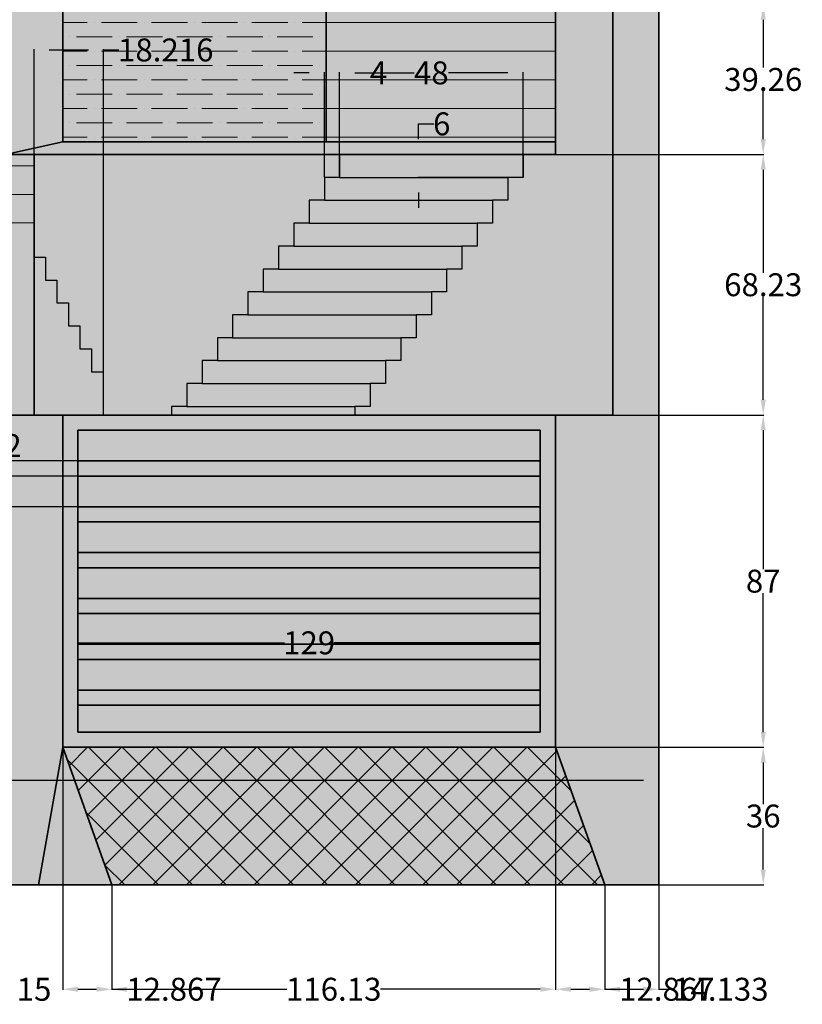
# Model space of a CAD drawing. Units: inches. Extents: x 184 to 649, y 215 to 818.
# Tile 3 of 9: x 442 to 647, y 215 to 473. Entities that reach past the tile are written whole.
import ezdxf

# ---------------------------------------------------------------- set-up
doc = ezdxf.new("R2010")
doc.units = ezdxf.units.IN
doc.header["$MEASUREMENT"] = 0
for name, color, linetype, lineweight in [('A-ANNO-DIMS', 2, 'Continuous', 18), ('A-ELEV', 7, 'Continuous', 35), ('A-ELEV-FILL', 9, 'Continuous', 13), ('A-ELEV-PATT', 8, 'Continuous', 13), ('A-FLOR-STRS', 3, 'Continuous', 25)]:
    doc.layers.add(name, color=color, linetype=linetype, lineweight=lineweight)
doc.styles.get("Standard").update_dxf_attribs({"font": 'arial.ttf'})
doc.dimstyles.get("Standard").update_dxf_attribs({"dimtxt": 6, "dimasz": 4, "dimexe": 0.18, "dimexo": 0.0625, "dimgap": 0.09, "dimtad": 0, "dimtih": 1, "dimtoh": 1, "dimdec": 0, "dimzin": 0, "dimdsep": 46, "dimlunit": 3, "dimtxsty": 'Standard', "dimcen": 0.09, "dimadec": 0, "dimazin": 0, "dimtfac": 1, "dimtdec": 0, "dimtofl": 0, "dimtmove": 0, "dimatfit": 3, "dimfxl": 1, "dimtolj": 1, "dimtzin": 0, "dimarcsym": 0})

# ---------------------------------------------------------------- blocks, each defined once
blk = doc.blocks.new('*D9')
at = {"layer": 'A-ANNO-DIMS', "color": 0, "lineweight": -2, "transparency": 16777216}
for p, q in [((248.97, 246.79), (248.97, 274.26)), ((252.97, 274.08), (422.27, 274.08)), ((604.97, 274.08), (435.68, 274.08)), ((608.97, 246.79), (608.97, 274.26))]:
    blk.add_line(p, q, dxfattribs=at)
at = {"layer": 'A-ANNO-DIMS', "color": 0, "transparency": 16777216}
for points in [[(252.97, 274.74), (252.97, 273.41), (248.97, 274.08)], [(604.97, 274.74), (604.97, 273.41), (608.97, 274.08)]]:
    blk.add_solid(points, dxfattribs=at)
at = {"layer": 'Defpoints', "color": 0, "transparency": 16777216}
for p in [(608.97, 274.08), (248.97, 246.73), (608.97, 246.73)]:
    blk.add_point(p, dxfattribs=at)
at = {"layer": 'A-ANNO-DIMS', "color": 0, "transparency": 16777216, "insert": (428.97, 274.08), "char_height": 6, "attachment_point": 5}
blk.add_mtext('\\A1;360', dxfattribs=at)
blk = doc.blocks.new('*D14')
at = {"layer": 'A-ANNO-DIMS', "color": 0, "lineweight": -2, "transparency": 16777216}
for p, q in [((452.97, 282.66), (452.97, 219.2)), ((437.97, 246.66), (437.97, 219.2)), ((433.97, 219.38), (429.97, 219.38)), ((456.97, 219.38), (460.97, 219.38))]:
    blk.add_line(p, q, dxfattribs=at)
at = {"layer": 'A-ANNO-DIMS', "color": 0, "transparency": 16777216}
for points in [[(433.97, 220.04), (433.97, 218.71), (437.97, 219.38)], [(456.97, 220.04), (456.97, 218.71), (452.97, 219.38)]]:
    blk.add_solid(points, dxfattribs=at)
at = {"layer": 'Defpoints', "color": 0, "transparency": 16777216}
for p in [(452.97, 282.73), (437.97, 246.73), (452.97, 219.38)]:
    blk.add_point(p, dxfattribs=at)
at = {"layer": 'A-ANNO-DIMS', "color": 0, "transparency": 16777216, "insert": (445.47, 219.38), "char_height": 6, "attachment_point": 5}
blk.add_mtext('\\A1;15', dxfattribs=at)
blk = doc.blocks.new('*D15')
at = {"layer": 'A-ANNO-DIMS', "color": 0, "lineweight": -2, "transparency": 16777216}
for p, q in [((452.97, 282.66), (452.97, 219.2)), ((465.84, 246.66), (465.84, 219.2)), ((456.97, 219.38), (461.84, 219.38)), ((465.84, 219.38), (469.84, 219.38))]:
    blk.add_line(p, q, dxfattribs=at)
at = {"layer": 'A-ANNO-DIMS', "color": 0, "transparency": 16777216}
for points in [[(456.97, 220.04), (456.97, 218.71), (452.97, 219.38)], [(461.84, 220.04), (461.84, 218.71), (465.84, 219.38)]]:
    blk.add_solid(points, dxfattribs=at)
at = {"layer": 'Defpoints', "color": 0, "transparency": 16777216}
for p in [(452.97, 282.73), (465.84, 246.73), (465.84, 219.38)]:
    blk.add_point(p, dxfattribs=at)
at = {"layer": 'A-ANNO-DIMS', "color": 0, "transparency": 16777216, "insert": (482.1, 219.38), "char_height": 6, "attachment_point": 5}
blk.add_mtext('\\A1;12.867', dxfattribs=at)
blk = doc.blocks.new('*D16')
at = {"layer": 'A-ANNO-DIMS', "color": 0, "lineweight": -2, "transparency": 16777216}
for p, q in [((581.97, 282.66), (581.97, 219.2)), ((465.84, 246.66), (465.84, 219.2)), ((469.84, 219.38), (511.64, 219.38)), ((577.97, 219.38), (536.17, 219.38))]:
    blk.add_line(p, q, dxfattribs=at)
at = {"layer": 'A-ANNO-DIMS', "color": 0, "transparency": 16777216}
for points in [[(469.84, 220.04), (469.84, 218.71), (465.84, 219.38)], [(577.97, 220.04), (577.97, 218.71), (581.97, 219.38)]]:
    blk.add_solid(points, dxfattribs=at)
at = {"layer": 'Defpoints', "color": 0, "transparency": 16777216}
for p in [(581.97, 282.73), (465.84, 246.73), (581.97, 219.38)]:
    blk.add_point(p, dxfattribs=at)
at = {"layer": 'A-ANNO-DIMS', "color": 0, "transparency": 16777216, "insert": (523.91, 219.38), "char_height": 6, "attachment_point": 5}
blk.add_mtext('\\A1;116.13', dxfattribs=at)
blk = doc.blocks.new('*D17')
at = {"layer": 'A-ANNO-DIMS', "color": 0, "lineweight": -2, "transparency": 16777216}
for p, q in [((581.97, 282.66), (581.97, 219.2)), ((594.84, 246.66), (594.84, 219.2)), ((585.97, 219.38), (590.84, 219.38)), ((594.84, 219.38), (598.84, 219.38))]:
    blk.add_line(p, q, dxfattribs=at)
at = {"layer": 'A-ANNO-DIMS', "color": 0, "transparency": 16777216}
for points in [[(585.97, 220.04), (585.97, 218.71), (581.97, 219.38)], [(590.84, 220.04), (590.84, 218.71), (594.84, 219.38)]]:
    blk.add_solid(points, dxfattribs=at)
at = {"layer": 'Defpoints', "color": 0, "transparency": 16777216}
for p in [(581.97, 282.73), (594.84, 246.73), (594.84, 219.38)]:
    blk.add_point(p, dxfattribs=at)
at = {"layer": 'A-ANNO-DIMS', "color": 0, "transparency": 16777216, "insert": (611.1, 219.38), "char_height": 6, "attachment_point": 5}
blk.add_mtext('\\A1;12.867', dxfattribs=at)
blk = doc.blocks.new('*D18')
at = {"layer": 'A-ANNO-DIMS', "color": 0, "lineweight": -2, "transparency": 16777216}
for p, q in [((594.84, 246.66), (594.84, 219.2)), ((608.97, 246.66), (608.97, 219.2)), ((598.84, 219.38), (604.97, 219.38)), ((608.97, 219.38), (612.97, 219.38))]:
    blk.add_line(p, q, dxfattribs=at)
at = {"layer": 'A-ANNO-DIMS', "color": 0, "transparency": 16777216}
for points in [[(598.84, 220.04), (598.84, 218.71), (594.84, 219.38)], [(604.97, 220.04), (604.97, 218.71), (608.97, 219.38)]]:
    blk.add_solid(points, dxfattribs=at)
at = {"layer": 'Defpoints', "color": 0, "transparency": 16777216}
for p in [(594.84, 246.73), (608.97, 246.73), (608.97, 219.38)]:
    blk.add_point(p, dxfattribs=at)
at = {"layer": 'A-ANNO-DIMS', "color": 0, "transparency": 16777216, "insert": (625.23, 219.38), "char_height": 6, "attachment_point": 5}
blk.add_mtext('\\A1;14.133', dxfattribs=at)
blk = doc.blocks.new('*D44')
at = {"layer": 'A-ANNO-DIMS', "color": 0, "lineweight": -2, "transparency": 16777216}
for p, q in [((582.04, 282.73), (636.5, 282.73)), ((636.32, 278.73), (636.32, 267.88)), ((636.32, 250.73), (636.32, 261.57)), ((594.9, 246.73), (636.5, 246.73))]:
    blk.add_line(p, q, dxfattribs=at)
at = {"layer": 'A-ANNO-DIMS', "color": 0, "transparency": 16777216}
for points in [[(635.66, 278.73), (636.99, 278.73), (636.32, 282.73)], [(635.66, 250.73), (636.99, 250.73), (636.32, 246.73)]]:
    blk.add_solid(points, dxfattribs=at)
at = {"layer": 'Defpoints', "color": 0, "transparency": 16777216}
for p in [(581.97, 282.73), (636.32, 282.73), (594.84, 246.73)]:
    blk.add_point(p, dxfattribs=at)
at = {"layer": 'A-ANNO-DIMS', "color": 0, "transparency": 16777216, "insert": (636.32, 264.73), "char_height": 6, "attachment_point": 5}
blk.add_mtext('\\A1;36', dxfattribs=at)
blk = doc.blocks.new('*D45')
at = {"layer": 'A-ANNO-DIMS', "color": 0, "lineweight": -2, "transparency": 16777216}
for p, q in [((582.04, 369.73), (636.5, 369.73)), ((636.32, 365.73), (636.32, 329.38)), ((636.32, 286.73), (636.32, 323.07)), ((582.04, 282.73), (636.5, 282.73))]:
    blk.add_line(p, q, dxfattribs=at)
at = {"layer": 'A-ANNO-DIMS', "color": 0, "transparency": 16777216}
for points in [[(635.66, 365.73), (636.99, 365.73), (636.32, 369.73)], [(635.66, 286.73), (636.99, 286.73), (636.32, 282.73)]]:
    blk.add_solid(points, dxfattribs=at)
at = {"layer": 'Defpoints', "color": 0, "transparency": 16777216}
for p in [(581.97, 369.73), (636.32, 369.73), (581.97, 282.73)]:
    blk.add_point(p, dxfattribs=at)
at = {"layer": 'A-ANNO-DIMS', "color": 0, "transparency": 16777216, "insert": (636.32, 326.23), "char_height": 6, "attachment_point": 5}
blk.add_mtext('\\A1;87', dxfattribs=at)
blk = doc.blocks.new('*D46')
at = {"layer": 'A-ANNO-DIMS', "color": 0, "lineweight": -2, "transparency": 16777216}
for p, q in [((582.04, 437.96), (636.5, 437.96)), ((636.32, 433.96), (636.32, 407)), ((636.32, 373.73), (636.32, 400.69)), ((582.04, 369.73), (636.5, 369.73))]:
    blk.add_line(p, q, dxfattribs=at)
at = {"layer": 'A-ANNO-DIMS', "color": 0, "transparency": 16777216}
for points in [[(635.66, 433.96), (636.99, 433.96), (636.32, 437.96)], [(635.66, 373.73), (636.99, 373.73), (636.32, 369.73)]]:
    blk.add_solid(points, dxfattribs=at)
at = {"layer": 'Defpoints', "color": 0, "transparency": 16777216}
for p in [(581.97, 437.96), (636.32, 437.96), (581.97, 369.73)]:
    blk.add_point(p, dxfattribs=at)
at = {"layer": 'A-ANNO-DIMS', "color": 0, "transparency": 16777216, "insert": (636.32, 403.84), "char_height": 6, "attachment_point": 5}
blk.add_mtext('\\A1;68.23', dxfattribs=at)
blk = doc.blocks.new('*D47')
at = {"layer": 'A-ANNO-DIMS', "color": 0, "lineweight": -2, "transparency": 16777216}
for p, q in [((561.04, 477.22), (636.5, 477.22)), ((636.32, 473.22), (636.32, 460.75)), ((636.32, 441.96), (636.32, 454.44)), ((582.04, 437.96), (636.5, 437.96))]:
    blk.add_line(p, q, dxfattribs=at)
at = {"layer": 'A-ANNO-DIMS', "color": 0, "transparency": 16777216}
for points in [[(635.66, 473.22), (636.99, 473.22), (636.32, 477.22)], [(635.66, 441.96), (636.99, 441.96), (636.32, 437.96)]]:
    blk.add_solid(points, dxfattribs=at)
at = {"layer": 'Defpoints', "color": 0, "transparency": 16777216}
for p in [(560.97, 477.22), (636.32, 477.22), (581.97, 437.96)]:
    blk.add_point(p, dxfattribs=at)
at = {"layer": 'A-ANNO-DIMS', "color": 0, "transparency": 16777216, "insert": (636.32, 457.59), "char_height": 6, "attachment_point": 5}
blk.add_mtext('\\A1;39.26', dxfattribs=at)
blk = doc.blocks.new('*D64')
at = {"layer": 'A-ANNO-DIMS', "color": 0, "lineweight": -2, "transparency": 16777216}
for p, q in [((445.47, 438.02), (445.47, 465.49)), ((449.47, 465.31), (459.69, 465.31)), ((463.69, 438.02), (463.69, 465.49)), ((463.69, 465.31), (467.69, 465.31))]:
    blk.add_line(p, q, dxfattribs=at)
at = {"layer": 'A-ANNO-DIMS', "color": 0, "transparency": 16777216}
for points in [[(449.47, 465.98), (449.47, 464.64), (445.47, 465.31)], [(459.69, 465.98), (459.69, 464.64), (463.69, 465.31)]]:
    blk.add_solid(points, dxfattribs=at)
at = {"layer": 'Defpoints', "color": 0, "transparency": 16777216}
for p in [(463.69, 465.31), (445.47, 437.96), (463.69, 437.96)]:
    blk.add_point(p, dxfattribs=at)
at = {"layer": 'A-ANNO-DIMS', "color": 0, "transparency": 16777216, "insert": (479.95, 465.31), "char_height": 6, "attachment_point": 5}
blk.add_mtext('\\A1;18.216', dxfattribs=at)
blk = doc.blocks.new('*D65')
at = {"layer": 'A-ANNO-DIMS', "color": 0, "lineweight": -2, "transparency": 16777216}
for p, q in [((525.46, 432.02), (525.46, 459.49)), ((529.46, 459.31), (544.94, 459.31)), ((569.46, 459.31), (553.97, 459.31)), ((573.46, 432.02), (573.46, 459.49))]:
    blk.add_line(p, q, dxfattribs=at)
at = {"layer": 'A-ANNO-DIMS', "color": 0, "transparency": 16777216}
for points in [[(529.46, 459.98), (529.46, 458.64), (525.46, 459.31)], [(569.46, 459.98), (569.46, 458.64), (573.46, 459.31)]]:
    blk.add_solid(points, dxfattribs=at)
at = {"layer": 'Defpoints', "color": 0, "transparency": 16777216}
for p in [(573.46, 459.31), (525.46, 431.96), (573.46, 431.96)]:
    blk.add_point(p, dxfattribs=at)
at = {"layer": 'A-ANNO-DIMS', "color": 0, "transparency": 16777216, "insert": (549.46, 459.31), "char_height": 6, "attachment_point": 5}
blk.add_mtext('\\A1;48', dxfattribs=at)
blk = doc.blocks.new('*D66')
at = {"layer": 'A-ANNO-DIMS', "color": 0, "lineweight": -2, "transparency": 16777216}
for p, q in [((517.46, 459.31), (513.46, 459.31)), ((521.46, 432.02), (521.46, 459.49)), ((525.46, 432.02), (525.46, 459.49)), ((529.46, 459.31), (533.46, 459.31))]:
    blk.add_line(p, q, dxfattribs=at)
at = {"layer": 'A-ANNO-DIMS', "color": 0, "transparency": 16777216}
for points in [[(517.46, 459.98), (517.46, 458.64), (521.46, 459.31)], [(529.46, 459.98), (529.46, 458.64), (525.46, 459.31)]]:
    blk.add_solid(points, dxfattribs=at)
at = {"layer": 'Defpoints', "color": 0, "transparency": 16777216}
for p in [(525.46, 459.31), (521.46, 431.96), (525.46, 431.96)]:
    blk.add_point(p, dxfattribs=at)
at = {"layer": 'A-ANNO-DIMS', "color": 0, "transparency": 16777216, "insert": (535.62, 459.31), "char_height": 6, "attachment_point": 5}
blk.add_mtext('\\A1;4', dxfattribs=at)
blk = doc.blocks.new('*D67')
at = {"layer": 'A-ANNO-DIMS', "color": 0, "lineweight": -2, "transparency": 16777216}
for p, q in [((546.11, 441.96), (546.11, 445.96)), ((546.11, 445.96), (550.11, 445.96)), ((573.4, 437.96), (545.93, 437.96)), ((573.4, 431.96), (545.93, 431.96)), ((546.11, 427.96), (546.11, 423.96))]:
    blk.add_line(p, q, dxfattribs=at)
at = {"layer": 'A-ANNO-DIMS', "color": 0, "transparency": 16777216}
for points in [[(545.44, 441.96), (546.77, 441.96), (546.11, 437.96)], [(545.44, 427.96), (546.77, 427.96), (546.11, 431.96)]]:
    blk.add_solid(points, dxfattribs=at)
at = {"layer": 'Defpoints', "color": 0, "transparency": 16777216}
for p in [(546.11, 437.96), (573.46, 437.96), (573.46, 431.96)]:
    blk.add_point(p, dxfattribs=at)
at = {"layer": 'A-ANNO-DIMS', "color": 0, "transparency": 16777216, "insert": (552.18, 445.96), "char_height": 6, "attachment_point": 5}
blk.add_mtext('\\A1;6', dxfattribs=at)
blk = doc.blocks.new('*D70')
at = {"layer": 'A-ANNO-DIMS', "color": 0, "lineweight": -2, "transparency": 16777216}
for p, q in [((452.97, 282.79), (452.97, 310.26)), ((456.97, 310.08), (511.03, 310.08)), ((577.97, 310.08), (523.91, 310.08)), ((581.97, 282.79), (581.97, 310.26))]:
    blk.add_line(p, q, dxfattribs=at)
at = {"layer": 'A-ANNO-DIMS', "color": 0, "transparency": 16777216}
for points in [[(456.97, 310.74), (456.97, 309.41), (452.97, 310.08)], [(577.97, 310.74), (577.97, 309.41), (581.97, 310.08)]]:
    blk.add_solid(points, dxfattribs=at)
at = {"layer": 'Defpoints', "color": 0, "transparency": 16777216}
for p in [(581.97, 310.08), (452.97, 282.73), (581.97, 282.73)]:
    blk.add_point(p, dxfattribs=at)
at = {"layer": 'A-ANNO-DIMS', "color": 0, "transparency": 16777216, "insert": (517.47, 310.08), "char_height": 6, "attachment_point": 5}
blk.add_mtext('\\A1;129', dxfattribs=at)
blk = doc.blocks.new('*D71')
at = {"layer": 'A-ANNO-DIMS', "color": 0, "lineweight": -2, "transparency": 16777216}
for p, q in [((429.62, 361.73), (429.62, 365.73)), ((429.62, 365.73), (433.62, 365.73)), ((456.91, 357.73), (429.44, 357.73)), ((456.91, 353.73), (429.44, 353.73)), ((429.62, 349.73), (429.62, 345.73))]:
    blk.add_line(p, q, dxfattribs=at)
at = {"layer": 'A-ANNO-DIMS', "color": 0, "transparency": 16777216}
for points in [[(428.96, 361.73), (430.29, 361.73), (429.62, 357.73)], [(428.96, 349.73), (430.29, 349.73), (429.62, 353.73)]]:
    blk.add_solid(points, dxfattribs=at)
at = {"layer": 'Defpoints', "color": 0, "transparency": 16777216}
for p in [(429.62, 357.73), (456.97, 357.73), (456.97, 353.73)]:
    blk.add_point(p, dxfattribs=at)
at = {"layer": 'A-ANNO-DIMS', "color": 0, "transparency": 16777216, "insert": (435.79, 365.73), "char_height": 6, "attachment_point": 5}
blk.add_mtext('\\A1;4', dxfattribs=at)
blk = doc.blocks.new('*D72')
at = {"layer": 'A-ANNO-DIMS', "color": 0, "lineweight": -2, "transparency": 16777216}
for p, q in [((429.62, 357.73), (429.62, 361.73)), ((429.62, 361.73), (433.62, 361.73)), ((456.91, 357.73), (429.44, 357.73)), ((429.62, 349.73), (429.62, 353.73)), ((456.91, 345.73), (429.44, 345.73))]:
    blk.add_line(p, q, dxfattribs=at)
at = {"layer": 'A-ANNO-DIMS', "color": 0, "transparency": 16777216}
for points in [[(428.96, 353.73), (430.29, 353.73), (429.62, 357.73)], [(428.96, 349.73), (430.29, 349.73), (429.62, 345.73)]]:
    blk.add_solid(points, dxfattribs=at)
at = {"layer": 'Defpoints', "color": 0, "transparency": 16777216}
for p in [(429.62, 357.73), (456.97, 357.73), (456.97, 345.73)]:
    blk.add_point(p, dxfattribs=at)
at = {"layer": 'A-ANNO-DIMS', "color": 0, "transparency": 16777216, "insert": (437.7, 361.73), "char_height": 6, "attachment_point": 5}
blk.add_mtext('\\A1;12', dxfattribs=at)

msp = doc.modelspace()

# ---------------------------------------------------------------- hatches: boundary and pattern name
at = {"layer": 'A-ELEV-FILL'}
h = msp.add_hatch(color=256, dxfattribs=at)
h.dxf.hatch_style = 1
h.paths.add_polyline_path([(452.9726, 369.7265), (248.9726, 369.7265), (248.9726, 246.7265), (275.9726, 246.7265), (275.9726, 328.7265), (437.9726, 328.7265), (437.9726, 246.7265), (446.6666, 246.7265), (452.9726, 282.7265)])
h.paths.add_polyline_path([(275.9726, 340.7265), (275.9726, 354.7265), (437.9726, 354.7265), (437.9726, 340.7265)], flags=16)
h.paths.add_polyline_path([(452.9726, 510.7265), (260.9726, 510.7265), (260.9726, 642.7265), (260.9726, 699.7265), (367.0226, 699.7265), (373.9381, 706.7265), (260.9726, 706.7265), (260.9726, 715.7265), (382.8295, 715.7265), (389.745, 722.7265), (260.9726, 722.7265), (260.9726, 731.7265), (398.6364, 731.7265), (405.5519, 738.7265), (260.9726, 738.7265), (260.9726, 747.7265), (414.4433, 747.7265), (421.3588, 754.7265), (260.9726, 754.7265), (260.9726, 763.7265), (430.2502, 763.7265), (437.1657, 770.7265), (260.9726, 770.7265), (260.9726, 779.7265), (446.057, 779.7265), (452.9726, 786.7265), (248.9726, 786.7265), (248.9726, 369.7265), (260.9726, 369.7265), (260.9726, 498.7265), (452.9726, 498.7265)])
h = msp.add_hatch(color=256, dxfattribs=at)
h.dxf.hatch_style = 1
h.paths.add_polyline_path([(608.9726, 786.7265), (452.9726, 786.7265), (360.1071, 692.7265), (372.3627, 692.7265), (452.9726, 774.7265), (596.9726, 774.7265), (596.9726, 369.7265), (581.9726, 369.7265), (581.9726, 282.7265), (594.8393, 246.7265), (608.9726, 246.7265)])
h = msp.add_hatch(color=256, dxfattribs=at)
h.dxf.hatch_style = 1
h.paths.add_polyline_path([(596.9726, 774.7265), (581.9726, 759.7265), (581.9726, 437.9607), (573.4578, 437.9607), (573.4578, 431.9607), (569.4578, 431.9607), (569.4578, 425.9607), (565.4578, 425.9607), (565.4578, 419.9607), (561.4578, 419.9607), (561.4578, 413.9607), (557.4578, 413.9607), (557.4578, 407.9607), (553.4578, 407.9607), (553.4578, 401.9607), (549.4578, 401.9607), (549.4578, 395.9607), (545.4578, 395.9607), (545.4578, 389.9607), (541.4578, 389.9607), (541.4578, 383.9607), (537.4578, 383.9607), (537.4578, 377.9607), (533.4578, 377.9607), (533.4578, 371.9607), (529.4578, 371.9607), (529.4578, 369.7265), (596.9726, 369.7265)])
h = msp.add_hatch(color=256, dxfattribs=at)
h.dxf.hatch_style = 1
h.paths.add_polyline_path([(380.9726, 453.5037), (422.2268, 453.5037), (422.2268, 474.7265), (260.9726, 474.7265), (260.9726, 369.7265), (291.9998, 369.7265), (291.9998, 453.5037), (339.9998, 453.5037), (339.9998, 369.7265), (380.9726, 369.7265)])
h.paths.add_polyline_path([(437.9726, 328.7265), (275.9726, 328.7265), (275.9726, 246.7265), (437.9726, 246.7265)])
h.paths.add_polyline_path([(581.9726, 759.7265), (521.9726, 759.7265), (521.9726, 441.2233), (581.9726, 441.2233)])
h.paths.add_polyline_path([(560.9726, 582.4749), (560.9726, 477.2233), (542.9726, 477.2233), (542.9726, 582.4749)], flags=16)
h.paths.add_polyline_path([(560.9726, 618.4749), (542.9726, 618.4749), (542.9726, 723.7265), (560.9726, 723.7265)], flags=16)
h = msp.add_hatch(color=256, dxfattribs=at)
h.dxf.hatch_style = 1
h.paths.add_polyline_path([(521.9726, 759.7265), (452.9726, 759.7265), (452.9726, 441.2233), (521.9726, 441.2233)])
h.paths.add_polyline_path([(491.9726, 477.2233), (476.9726, 477.2233), (476.9726, 723.7265), (491.9726, 723.7265)], flags=16)
h = msp.add_hatch(color=256, dxfattribs=at)
h.dxf.hatch_style = 1
h.paths.add_polyline_path([(437.9726, 498.7265), (260.9726, 498.7265), (260.9726, 474.7265), (422.2268, 474.7265), (422.2268, 453.5037), (428.9726, 453.5037), (428.9726, 417.0753), (445.4726, 417.0753), (445.4726, 437.9607), (437.9726, 437.9607)])
h = msp.add_hatch(color=256, dxfattribs=at)
h.dxf.hatch_style = 1
h.paths.add_polyline_path([(452.9726, 498.7265), (437.9726, 498.7265), (437.9726, 437.9607), (452.9726, 441.2233)])
h = msp.add_hatch(color=256, dxfattribs=at)
h.dxf.hatch_style = 1
h.paths.add_polyline_path([(581.9726, 441.2233), (452.9726, 441.2233), (437.9726, 437.9607), (581.9726, 437.9607)])
h = msp.add_hatch(color=256, dxfattribs=at)
h.dxf.hatch_style = 1
h.paths.add_polyline_path([(463.6889, 437.9607), (445.4726, 437.9607), (445.4726, 411.0753), (448.4726, 411.0753), (448.4726, 405.0753), (451.4726, 405.0753), (451.4726, 399.0753), (454.4726, 399.0753), (454.4726, 393.0753), (457.4726, 393.0753), (457.4726, 387.0753), (460.4726, 387.0753), (460.4726, 381.0753), (463.6889, 381.0753)])
h = msp.add_hatch(color=256, dxfattribs=at)
h.dxf.hatch_style = 1
h.paths.add_polyline_path([(501.4578, 401.9607), (505.4578, 401.9607), (505.4578, 407.9607), (509.4578, 407.9607), (509.4578, 413.9607), (513.4578, 413.9607), (513.4578, 419.9607), (517.4578, 419.9607), (517.4578, 425.9607), (521.4578, 425.9607), (521.4578, 431.9607), (525.4578, 431.9607), (525.4578, 437.9607), (463.6889, 437.9607), (463.6889, 369.7265), (481.4578, 369.7265), (481.4578, 371.9607), (485.4578, 371.9607), (485.4578, 377.9607), (489.4578, 377.9607), (489.4578, 383.9607), (493.4578, 383.9607), (493.4578, 389.9607), (497.4578, 389.9607), (497.4578, 395.9607), (501.4578, 395.9607)])
h = msp.add_hatch(color=256, dxfattribs=at)
h.dxf.hatch_style = 1
h.paths.add_polyline_path([(573.4578, 437.9607), (525.4578, 437.9607), (525.4578, 431.9607), (569.4578, 431.9607), (573.4578, 431.9607)])
h.paths.add_polyline_path([(569.4578, 431.9607), (525.4578, 431.9607), (521.4578, 431.9607), (521.4578, 425.9607), (565.4578, 425.9607), (569.4578, 425.9607)])
h.paths.add_polyline_path([(565.4578, 425.9607), (521.4578, 425.9607), (517.4578, 425.9607), (517.4578, 419.9607), (561.4578, 419.9607), (565.4578, 419.9607)])
h.paths.add_polyline_path([(561.4578, 419.9607), (517.4578, 419.9607), (513.4578, 419.9607), (513.4578, 413.9607), (557.4578, 413.9607), (561.4578, 413.9607)])
h.paths.add_polyline_path([(557.4578, 413.9607), (513.4578, 413.9607), (509.4578, 413.9607), (509.4578, 407.9607), (553.4578, 407.9607), (557.4578, 407.9607)])
h.paths.add_polyline_path([(553.4578, 407.9607), (509.4578, 407.9607), (505.4578, 407.9607), (505.4578, 401.9607), (549.4578, 401.9607), (553.4578, 401.9607)])
h.paths.add_polyline_path([(549.4578, 401.9607), (505.4578, 401.9607), (501.4578, 401.9607), (501.4578, 395.9607), (545.4578, 395.9607), (549.4578, 395.9607)])
h.paths.add_polyline_path([(545.4578, 395.9607), (501.4578, 395.9607), (497.4578, 395.9607), (497.4578, 389.9607), (541.4578, 389.9607), (545.4578, 389.9607)])
h.paths.add_polyline_path([(529.4578, 371.9607), (485.4578, 371.9607), (481.4578, 371.9607), (481.4578, 369.7265), (529.4578, 369.7265)])
h.paths.add_polyline_path([(533.4578, 377.9607), (489.4578, 377.9607), (485.4578, 377.9607), (485.4578, 371.9607), (529.4578, 371.9607), (533.4578, 371.9607)])
h.paths.add_polyline_path([(537.4578, 383.9607), (493.4578, 383.9607), (489.4578, 383.9607), (489.4578, 377.9607), (533.4578, 377.9607), (537.4578, 377.9607)])
h.paths.add_polyline_path([(541.4578, 389.9607), (497.4578, 389.9607), (493.4578, 389.9607), (493.4578, 383.9607), (537.4578, 383.9607), (541.4578, 383.9607)])
h = msp.add_hatch(color=256, dxfattribs=at)
h.dxf.hatch_style = 1
h.paths.add_polyline_path([(445.4726, 417.0753), (428.9726, 417.0753), (428.9726, 369.7265), (445.4726, 369.7265)])
h = msp.add_hatch(color=256, dxfattribs=at)
h.dxf.hatch_style = 1
h.paths.add_polyline_path([(445.4726, 369.7265), (463.6889, 369.7265), (463.6889, 381.0753), (463.4726, 381.0753), (460.4726, 381.0753), (460.4726, 387.0753), (457.4726, 387.0753), (457.4726, 393.0753), (454.4726, 393.0753), (454.4726, 399.0753), (451.4726, 399.0753), (451.4726, 405.0753), (448.4726, 405.0753), (448.4726, 411.0753), (445.4726, 411.0753)])
h = msp.add_hatch(color=256, dxfattribs=at)
h.dxf.hatch_style = 1
h.paths.add_polyline_path([(452.9726, 369.7265), (452.9726, 282.7265), (581.9726, 282.7265), (581.9726, 369.7265)])
h.paths.add_polyline_path([(577.9726, 365.7265), (577.9726, 286.7265), (456.9726, 286.7265), (456.9726, 365.7265)], flags=16)
h = msp.add_hatch(color=256, dxfattribs=at)
h.dxf.hatch_style = 1
h.paths.add_polyline_path([(456.9726, 293.7265), (456.9726, 286.7265), (577.9726, 286.7265), (577.9726, 293.7265)])
h.paths.add_polyline_path([(577.9726, 297.7265), (577.9726, 305.7265), (456.9726, 305.7265), (456.9726, 297.7265)])
h.paths.add_polyline_path([(456.9726, 317.7265), (456.9726, 309.7265), (577.9726, 309.7265), (577.9726, 317.7265)])
h.paths.add_polyline_path([(577.9726, 321.7265), (577.9726, 329.7265), (456.9726, 329.7265), (456.9726, 321.7265)])
h.paths.add_polyline_path([(456.9726, 341.7265), (456.9726, 333.7265), (577.9726, 333.7265), (577.9726, 341.7265)])
h.paths.add_polyline_path([(577.9726, 345.7265), (577.9726, 353.7265), (456.9726, 353.7265), (456.9726, 345.7265)])
h.paths.add_polyline_path([(456.9726, 365.7265), (456.9726, 357.7265), (577.9726, 357.7265), (577.9726, 365.7265)])
h = msp.add_hatch(color=256, dxfattribs=at)
h.dxf.hatch_style = 1
h.paths.add_polyline_path([(577.9726, 362.7265), (456.9726, 362.7265), (456.9726, 360.7265), (577.9726, 360.7265)])
h.paths.add_polyline_path([(577.9726, 350.7265), (456.9726, 350.7265), (456.9726, 348.7265), (577.9726, 348.7265)])
h.paths.add_polyline_path([(577.9726, 338.7265), (456.9726, 338.7265), (456.9726, 336.7265), (577.9726, 336.7265)])
h.paths.add_polyline_path([(577.9726, 326.7265), (456.9726, 326.7265), (456.9726, 324.7265), (577.9726, 324.7265)])
h.paths.add_polyline_path([(577.9726, 314.7265), (456.9726, 314.7265), (456.9726, 312.7265), (577.9726, 312.7265)])
h.paths.add_polyline_path([(577.9726, 302.7265), (456.9726, 302.7265), (456.9726, 300.7265), (577.9726, 300.7265)])
h.paths.add_polyline_path([(577.9726, 291.2265), (456.9726, 291.2265), (456.9726, 289.2265), (577.9726, 289.2265)])
h = msp.add_hatch(color=256, dxfattribs=at)
h.dxf.hatch_style = 1
h.paths.add_polyline_path([(577.9726, 353.7265), (577.9726, 357.7265), (456.9726, 357.7265), (456.9726, 353.7265)])
h.paths.add_polyline_path([(456.9726, 345.7265), (456.9726, 341.7265), (577.9726, 341.7265), (577.9726, 345.7265)])
h.paths.add_polyline_path([(456.9726, 333.7265), (456.9726, 329.7265), (577.9726, 329.7265), (577.9726, 333.7265)])
h.paths.add_polyline_path([(456.9726, 321.7265), (456.9726, 317.7265), (577.9726, 317.7265), (577.9726, 321.7265)])
h.paths.add_polyline_path([(456.9726, 309.7265), (456.9726, 305.7265), (577.9726, 305.7265), (577.9726, 309.7265)])
h.paths.add_polyline_path([(577.9726, 293.7265), (577.9726, 297.7265), (456.9726, 297.7265), (456.9726, 293.7265)])
h = msp.add_hatch(color=256, dxfattribs=at)
h.dxf.hatch_style = 1
h.paths.add_polyline_path([(452.9726, 282.7265), (446.6666, 246.7265), (465.8393, 246.7265)])
h = msp.add_hatch(color=256, dxfattribs=at)
h.dxf.hatch_style = 1
h.paths.add_polyline_path([(581.9726, 282.7265), (452.9726, 282.7265), (465.8393, 246.7265), (594.8393, 246.7265)])
at = {"layer": 'A-ELEV-PATT'}
h = msp.add_hatch(dxfattribs=at)
h.set_pattern_fill('ANSI36', color=256, scale=30, angle=135)
h.paths.add_polyline_path([(521.9726, 759.7265), (452.9726, 759.7265), (452.9726, 441.2233), (521.9726, 441.2233)])
h.paths.add_polyline_path([(476.9726, 723.7265), (491.9726, 723.7265), (491.9726, 477.2233), (476.9726, 477.2233)], flags=16)
h = msp.add_hatch(dxfattribs=at)
h.set_pattern_fill('ANSI31', color=256, scale=60, angle=135)
h.paths.add_polyline_path([(581.9726, 759.7265), (521.9726, 759.7265), (521.9726, 441.2233), (581.9726, 441.2233)])
h.paths.add_polyline_path([(560.9726, 723.7265), (560.9726, 618.4749), (542.9726, 618.4749), (542.9726, 723.7265)], flags=16)
h.paths.add_polyline_path([(560.9726, 582.4749), (560.9726, 477.2233), (542.9726, 477.2233), (542.9726, 582.4749)], flags=16)
h = msp.add_hatch(dxfattribs=at)
h.set_pattern_fill('ANSI31', color=256, scale=60, angle=135)
h.paths.add_polyline_path([(437.9726, 498.7265), (260.9726, 498.7265), (260.9726, 369.7265), (291.9998, 369.7265), (291.9998, 453.5037), (339.9998, 453.5037), (339.9998, 369.7265), (380.9726, 369.7265), (380.9726, 453.5037), (428.9726, 453.5037), (428.9726, 417.0753), (445.4726, 417.0753), (445.4726, 437.9607), (437.9726, 437.9607)])
h = msp.add_hatch(dxfattribs=at)
h.set_pattern_fill('ANSI37', color=256, scale=50, angle=90)
h.paths.add_polyline_path([(581.9726, 282.7265), (452.9726, 282.7265), (465.8393, 246.7265), (594.8393, 246.7265)])

# ---------------------------------------------------------------- linework, layer by layer
at = {"layer": 'A-ELEV'}
for p, q in [((608.9726, 246.7265), (608.9726, 786.7265)), ((596.9726, 369.7265), (596.9726, 774.7265)), ((452.9726, 441.2233), (452.9726, 759.7265)), ((521.9726, 441.2233), (521.9726, 759.7265)), ((581.9726, 437.9607), (581.9726, 759.7265)), ((452.9726, 441.2233), (437.9726, 437.9607)), ((452.9726, 441.2233), (581.9726, 441.2233)), ((437.9726, 437.9607), (581.9726, 437.9607)), ((445.4726, 369.7265), (445.4726, 437.9607)), ((445.4726, 417.0753), (445.4726, 411.0753)), ((596.9726, 369.7265), (248.9726, 369.7265)), ((452.9726, 369.7265), (452.9726, 282.7265)), ((581.9726, 282.7265), (581.9726, 369.7265)), ((456.9726, 365.7265), (456.9726, 286.7265)), ((577.9726, 365.7265), (456.9726, 365.7265)), ((577.9726, 286.7265), (577.9726, 365.7265)), ((577.9726, 357.7265), (456.9726, 357.7265)), ((577.9726, 353.7265), (456.9726, 353.7265)), ((577.9726, 345.7265), (456.9726, 345.7265)), ((577.9726, 341.7265), (456.9726, 341.7265)), ((577.9726, 333.7265), (456.9726, 333.7265)), ((577.9726, 329.7265), (456.9726, 329.7265)), ((577.9726, 321.7265), (456.9726, 321.7265)), ((577.9726, 317.7265), (456.9726, 317.7265)), ((577.9726, 309.7265), (456.9726, 309.7265)), ((577.9726, 305.7265), (456.9726, 305.7265)), ((577.9726, 297.7265), (456.9726, 297.7265)), ((577.9726, 293.7265), (456.9726, 293.7265)), ((577.9726, 286.7265), (456.9726, 286.7265)), ((452.9726, 282.7265), (446.6666, 246.7265)), ((581.9726, 282.7265), (452.9726, 282.7265)), ((452.9726, 282.7265), (465.8393, 246.7265)), ((581.9726, 282.7265), (594.8393, 246.7265)), ((248.9726, 246.7265), (608.9726, 246.7265))]:
    msp.add_line(p, q, dxfattribs=at)
at = {"layer": 'A-FLOR-STRS'}
for p, q in [((463.6889, 369.7265), (463.6889, 437.9607)), ((525.4578, 437.9607), (525.4578, 431.9607)), ((573.4578, 437.9607), (573.4578, 431.9607)), ((525.4578, 431.9607), (521.4578, 431.9607)), ((521.4578, 431.9607), (521.4578, 425.9607)), ((525.4578, 431.9607), (569.4578, 431.9607)), ((573.4578, 431.9607), (569.4578, 431.9607)), ((569.4578, 431.9607), (569.4578, 425.9607)), ((521.4578, 425.9607), (517.4578, 425.9607)), ((517.4578, 425.9607), (517.4578, 419.9607)), ((521.4578, 425.9607), (565.4578, 425.9607)), ((569.4578, 425.9607), (565.4578, 425.9607)), ((565.4578, 425.9607), (565.4578, 419.9607)), ((517.4578, 419.9607), (513.4578, 419.9607)), ((513.4578, 419.9607), (513.4578, 413.9607)), ((517.4578, 419.9607), (561.4578, 419.9607)), ((565.4578, 419.9607), (561.4578, 419.9607)), ((561.4578, 419.9607), (561.4578, 413.9607)), ((513.4578, 413.9607), (509.4578, 413.9607)), ((509.4578, 413.9607), (509.4578, 407.9607)), ((513.4578, 413.9607), (557.4578, 413.9607)), ((561.4578, 413.9607), (557.4578, 413.9607)), ((557.4578, 413.9607), (557.4578, 407.9607)), ((445.4726, 411.0753), (448.4726, 411.0753)), ((448.4726, 411.0753), (448.4726, 405.0753)), ((509.4578, 407.9607), (505.4578, 407.9607)), ((505.4578, 407.9607), (505.4578, 401.9607)), ((509.4578, 407.9607), (553.4578, 407.9607)), ((557.4578, 407.9607), (553.4578, 407.9607)), ((553.4578, 407.9607), (553.4578, 401.9607)), ((448.4726, 405.0753), (451.4726, 405.0753)), ((451.4726, 405.0753), (451.4726, 399.0753)), ((505.4578, 401.9607), (501.4578, 401.9607)), ((501.4578, 401.9607), (501.4578, 395.9607)), ((505.4578, 401.9607), (549.4578, 401.9607)), ((553.4578, 401.9607), (549.4578, 401.9607)), ((549.4578, 401.9607), (549.4578, 395.9607)), ((451.4726, 399.0753), (454.4726, 399.0753)), ((454.4726, 399.0753), (454.4726, 393.0753)), ((501.4578, 395.9607), (497.4578, 395.9607)), ((497.4578, 395.9607), (497.4578, 389.9607)), ((501.4578, 395.9607), (545.4578, 395.9607)), ((549.4578, 395.9607), (545.4578, 395.9607)), ((545.4578, 395.9607), (545.4578, 389.9607)), ((454.4726, 393.0753), (457.4726, 393.0753)), ((457.4726, 393.0753), (457.4726, 387.0753)), ((497.4578, 389.9607), (493.4578, 389.9607)), ((493.4578, 389.9607), (493.4578, 383.9607)), ((497.4578, 389.9607), (541.4578, 389.9607)), ((545.4578, 389.9607), (541.4578, 389.9607)), ((541.4578, 389.9607), (541.4578, 383.9607)), ((457.4726, 387.0753), (460.4726, 387.0753)), ((460.4726, 387.0753), (460.4726, 381.0753)), ((493.4578, 383.9607), (489.4578, 383.9607)), ((489.4578, 383.9607), (489.4578, 377.9607)), ((493.4578, 383.9607), (537.4578, 383.9607)), ((541.4578, 383.9607), (537.4578, 383.9607)), ((537.4578, 383.9607), (537.4578, 377.9607)), ((460.4726, 381.0753), (463.4726, 381.0753)), ((463.4726, 381.0753), (463.6889, 381.0753)), ((489.4578, 377.9607), (485.4578, 377.9607)), ((485.4578, 377.9607), (485.4578, 371.9607)), ((489.4578, 377.9607), (533.4578, 377.9607)), ((537.4578, 377.9607), (533.4578, 377.9607)), ((533.4578, 377.9607), (533.4578, 371.9607)), ((485.4578, 371.9607), (481.4578, 371.9607)), ((481.4578, 371.9607), (481.4578, 369.7265)), ((485.4578, 371.9607), (529.4578, 371.9607)), ((533.4578, 371.9607), (529.4578, 371.9607)), ((529.4578, 371.9607), (529.4578, 369.7265))]:
    msp.add_line(p, q, dxfattribs=at)

# ---------------------------------------------------------------- dimensions: what is measured, and where the dimension line sits
at = {"layer": 'A-ANNO-DIMS'}
for base, p1, p2, angle, override, picture, middle in [((636.3226, 477.2233), (581.9726, 437.9607), (560.9726, 477.2233), 90, {"dimdec": 2, "dimlfac": 1, "dimrnd": 0, "dimzin": 0, "dimdsep": 46, "dimlunit": 2}, '*D47', (636.3226, 457.592)), ((463.6889, 465.3107), (445.4726, 437.9607), (463.6889, 437.9607), 0, {"dimdec": 3, "dimlfac": 1, "dimrnd": 0, "dimzin": 0, "dimdsep": 46, "dimlunit": 2}, '*D64', (479.9487, 465.3107)), ((546.1078, 437.9607), (573.4578, 431.9607), (573.4578, 437.9607), 90, {"dimdec": 0, "dimlfac": 1, "dimrnd": 0, "dimzin": 0, "dimdsep": 46, "dimlunit": 2}, '*D67', (552.1787, 445.9607)), ((636.3226, 437.9607), (581.9726, 369.7265), (581.9726, 437.9607), 90, {"dimdec": 2, "dimlfac": 1, "dimrnd": 0, "dimzin": 0, "dimdsep": 46, "dimlunit": 2}, '*D46', (636.3226, 403.8436)), ((429.6226, 357.7265), (456.9726, 353.7265), (456.9726, 357.7265), 90, {"dimdec": 0, "dimlfac": 1, "dimrnd": 0, "dimzin": 0, "dimdsep": 46, "dimlunit": 2}, '*D71', (435.7876, 365.7265)), ((636.3226, 369.7265), (581.9726, 282.7265), (581.9726, 369.7265), 90, {"dimdec": 0, "dimlfac": 1, "dimrnd": 0, "dimzin": 0, "dimdsep": 46, "dimlunit": 2}, '*D45', (636.3226, 326.2265)), ((429.6226, 357.7265), (456.9726, 345.7265), (456.9726, 357.7265), 90, {"dimdec": 0, "dimlfac": 1, "dimrnd": 0, "dimzin": 0, "dimdsep": 46, "dimlunit": 2}, '*D72', (437.6969, 361.7265)), ((636.3226, 282.7265), (594.8393, 246.7265), (581.9726, 282.7265), 90, {"dimdec": 0, "dimlfac": 1, "dimrnd": 0, "dimzin": 0, "dimdsep": 46, "dimlunit": 2}, '*D44', (636.3226, 264.7265))]:
    dim = msp.add_linear_dim(base=base, p1=p1, p2=p2, angle=angle, dimstyle='Standard', override=override, dxfattribs=at)
    dim.commit()
    dim.dimension.update_dxf_attribs({"geometry": picture, "text_midpoint": middle})
for base, p1, p2, override, picture, middle in [((525.4578, 459.3107), (521.4578, 431.9607), (525.4578, 431.9607), {"dimdec": 0, "dimlfac": 1, "dimrnd": 0, "dimzin": 0, "dimdsep": 46, "dimlunit": 2}, '*D66', (535.6228, 459.3107)), ((573.4578, 459.3107), (525.4578, 431.9607), (573.4578, 431.9607), {"dimdec": 0, "dimlfac": 1, "dimrnd": 0, "dimzin": 0, "dimdsep": 46, "dimlunit": 2}, '*D65', (549.4578, 459.3107)), ((581.9726, 310.0765), (452.9726, 282.7265), (581.9726, 282.7265), {"dimdec": 0, "dimlfac": 1, "dimrnd": 0, "dimzin": 0, "dimdsep": 46, "dimlunit": 2}, '*D70', (517.4726, 310.0765)), ((452.9726, 219.3765), (437.9726, 246.7265), (452.9726, 282.7265), {"dimdec": 0, "dimlfac": 1, "dimrnd": 0, "dimzin": 0, "dimdsep": 46, "dimlunit": 2}, '*D14', (445.4726, 219.3765)), ((465.8393, 219.3765), (452.9726, 282.7265), (465.8393, 246.7265), {"dimdec": 3, "dimlfac": 1, "dimrnd": 0, "dimzin": 0, "dimdsep": 46, "dimlunit": 2}, '*D15', (482.1012, 219.3765)), ((581.9726, 219.3765), (465.8393, 246.7265), (581.9726, 282.7265), {"dimdec": 2, "dimlfac": 1, "dimrnd": 0, "dimzin": 0, "dimdsep": 46, "dimlunit": 2}, '*D16', (523.9059, 219.3765)), ((594.8393, 219.3765), (581.9726, 282.7265), (594.8393, 246.7265), {"dimdec": 3, "dimlfac": 1, "dimrnd": 0, "dimzin": 0, "dimdsep": 46, "dimlunit": 2}, '*D17', (611.1012, 219.3765)), ((608.9726, 274.0765), (248.9726, 246.7265), (608.9726, 246.7265), {"dimdec": 0, "dimlfac": 1, "dimrnd": 0, "dimzin": 0, "dimdsep": 46, "dimlunit": 2}, '*D9', (428.9726, 274.0765)), ((608.9726, 219.3765), (594.8393, 246.7265), (608.9726, 246.7265), {"dimdec": 3, "dimlfac": 1, "dimrnd": 0, "dimzin": 0, "dimdsep": 46, "dimlunit": 2}, '*D18', (625.2345, 219.3765))]:
    dim = msp.add_linear_dim(base=base, p1=p1, p2=p2, dimstyle='Standard', override=override, dxfattribs=at)
    dim.commit()
    dim.dimension.update_dxf_attribs({"geometry": picture, "text_midpoint": middle})

doc.saveas('drawing.dxf')
